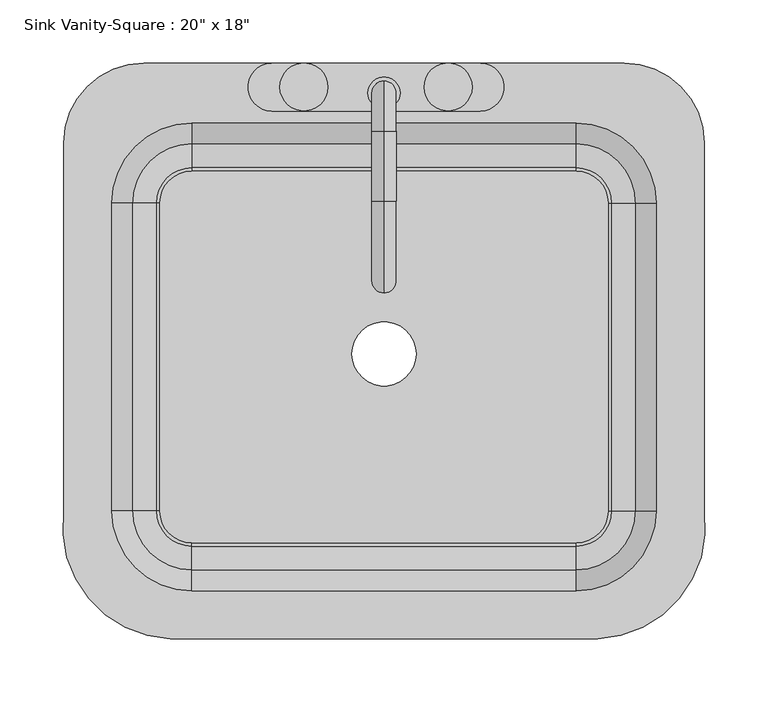
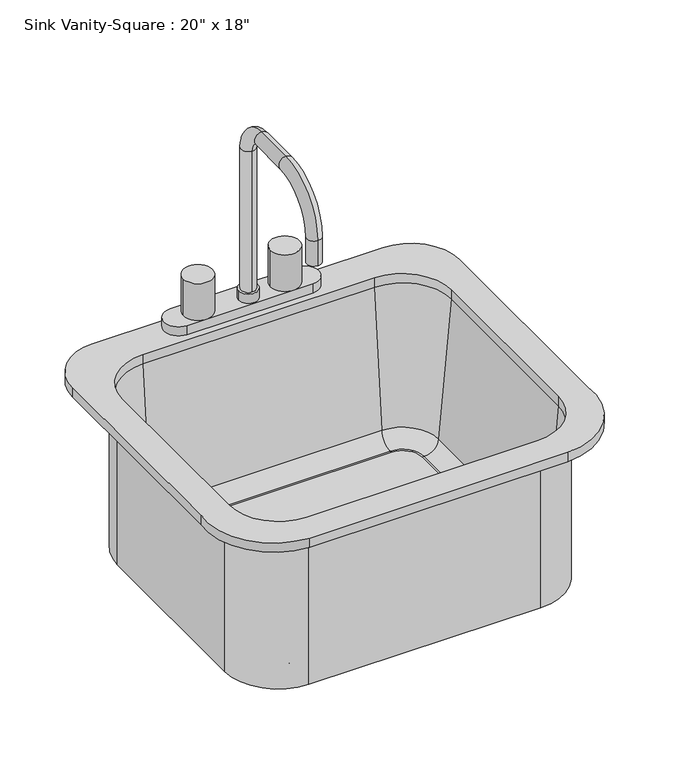
"""IFC4 building model written with IfcOpenShell, lengths in millimetres: flow terminal geometry."""

from ifc_helpers import new_model, si_unit, point, frame, frame_2d, origin, place, context, project, spatial, polyline, circle_curve, ellipse_curve, trimmed, segment, composite_curve, outline, extrude, source, transform, mapped, element, save
from ifc_brep_helpers import plane_surface, cylinder_surface, revolved_surface, advanced_brep


def flow_terminal_8d9ea526(model_context):
    return source(origin(), model_context, "Body", "SolidModel", [
        extrude(outline(composite_curve([segment(trimmed(circle_curve(frame_2d((168.0892406, 69.0204011)), 25.4), [point((168.0892406, 94.4204011))], [point((193.4892406, 69.0204011))], False, "CARTESIAN"), True, "CONTINUOUS"), segment(polyline([(193.4892406, 69.0204011), (193.4892406, -175.4545989)]), True, "CONTINUOUS"), segment(trimmed(circle_curve(frame_2d((168.0892406, -175.4545989)), 25.4), [point((193.4892406, -175.4545989))], [point((168.0892406, -200.8545989))], False, "CARTESIAN"), True, "CONTINUOUS"), segment(polyline([(168.0892406, -200.8545989), (-136.7107594, -200.8545989)]), True, "CONTINUOUS"), segment(trimmed(circle_curve(frame_2d((-136.7107594, -175.4545989)), 25.4), [point((-136.7107594, -200.8545989))], [point((-162.1107594, -175.4545989))], False, "CARTESIAN"), True, "CONTINUOUS"), segment(polyline([(-162.1107594, -175.4545989), (-162.1107594, 69.0204011)]), True, "CONTINUOUS"), segment(trimmed(circle_curve(frame_2d((-136.7107594, 69.0204011)), 25.4), [point((-162.1107594, 69.0204011))], [point((-136.7107594, 94.4204011))], False, "CARTESIAN"), True, "CONTINUOUS"), segment(polyline([(-136.7107594, 94.4204011), (168.0892406, 94.4204011)]), True, "CONTINUOUS")], self_intersect=False), holes=[composite_curve([segment(trimmed(circle_curve(frame_2d((15.6892406, -50.8)), 25.4), [point((-9.7107594, -50.8))], [point((41.0892406, -50.8))], True, "CARTESIAN"), True, "CONTINUOUS"), segment(trimmed(circle_curve(frame_2d((15.6892406, -50.8)), 25.4), [point((41.0892406, -50.8))], [point((-9.7107594, -50.8))], True, "CARTESIAN"), True, "CONTINUOUS")], self_intersect=False)]), frame((0.0, 0.0, 571.5), z_axis=(0.0, 0.0, 1.0), x_axis=(1.0, 0.0, 0.0)), (0.0, 0.0, 1.0), 9.525),
        extrude(outline(composite_curve([segment(trimmed(circle_curve(frame_2d((-47.8107594, 161.0954011)), 19.05), [point((-66.8607594, 161.0954011))], [point((-28.7607594, 161.0954011))], False, "CARTESIAN"), True, "CONTINUOUS"), segment(trimmed(circle_curve(frame_2d((-47.8107594, 161.0954011)), 19.05), [point((-28.7607594, 161.0954011))], [point((-66.8607594, 161.0954011))], False, "CARTESIAN"), True, "CONTINUOUS")], self_intersect=False)), frame((0.0, 0.0, 812.8), z_axis=(0.0, 0.0, 1.0), x_axis=(1.0, 0.0, 0.0)), (0.0, 0.0, 1.0), 50.8),
        extrude(outline(composite_curve([segment(trimmed(circle_curve(frame_2d((66.4892406, 161.0954011)), 19.05), [point((47.4392406, 161.0954011))], [point((85.5392406, 161.0954011))], False, "CARTESIAN"), True, "CONTINUOUS"), segment(trimmed(circle_curve(frame_2d((66.4892406, 161.0954011)), 19.05), [point((85.5392406, 161.0954011))], [point((47.4392406, 161.0954011))], False, "CARTESIAN"), True, "CONTINUOUS")], self_intersect=False)), frame((0.0, 0.0, 812.8), z_axis=(0.0, 0.0, 1.0), x_axis=(1.0, 0.0, 0.0)), (0.0, 0.0, 1.0), 50.8),
        advanced_brep(
        [(91.8892406, 180.1454011, 800.1), (91.8892406, 142.0454011, 800.1), (-73.2107594, 142.0454011, 800.1), (-73.2107594, 180.1454011, 800.1), (15.6892406, 165.8579011, 1020.7625), (15.6892406, 146.8079011, 1020.7625), (15.6892406, 146.8079011, 825.5), (15.6892406, 165.8579011, 825.5), (15.6892406, 126.1704011, 1060.45), (15.6892406, 126.1704011, 1041.4), (15.6892406, 70.6079011, 1060.45), (15.6892406, 70.6079011, 1041.4), (15.6892406, -2.4170989, 987.425), (15.6892406, 16.6329011, 987.425), (15.6892406, -2.4170989, 952.5), (15.6892406, 16.6329011, 952.5), (2.9892406, 156.3329011, 825.5), (28.3892406, 156.3329011, 825.5), (2.9892406, 156.3329011, 812.8), (28.3892406, 156.3329011, 812.8), (91.8892406, 180.1454011, 812.8), (-73.2107594, 180.1454011, 812.8), (-73.2107594, 142.0454011, 812.8), (91.8892406, 142.0454011, 812.8)],
        [
            (0, 1, circle_curve(frame((91.8892406, 161.0954011, 800.1), z_axis=(0.0, 0.0, -1.0), x_axis=(1.0, 0.0, 0.0)), 19.05)),
            (1, 2),
            (2, 3, circle_curve(frame((-73.2107594, 161.0954011, 800.1), z_axis=(0.0, 0.0, -1.0), x_axis=(1.0, 0.0, 0.0)), 19.05)),
            (3, 0),
            (4, 5, circle_curve(frame((15.6892406, 156.3329011, 1020.7625), z_axis=(0.0, 0.0, -1.0), x_axis=(0.0, -1.0, 0.0)), 9.525)),
            (5, 6),
            (6, 7, circle_curve(frame((15.6892406, 156.3329011, 825.5), z_axis=(0.0, 0.0, 1.0), x_axis=(0.0, -1.0, 0.0)), 9.525)),
            (7, 4),
            (5, 4, circle_curve(frame((15.6892406, 156.3329011, 1020.7625), z_axis=(0.0, 0.0, -1.0), x_axis=(0.0, -1.0, 0.0)), 9.525)),
            (7, 6, circle_curve(frame((15.6892406, 156.3329011, 825.5), z_axis=(0.0, 0.0, 1.0), x_axis=(0.0, -1.0, 0.0)), 9.525)),
            (4, 8, circle_curve(frame((15.6892406, 126.1704011, 1020.7625), z_axis=(1.0, 0.0, 0.0), x_axis=(0.0, 1.0, 0.0)), 39.6875)),
            (8, 9, circle_curve(frame((15.6892406, 126.1704011, 1050.925), z_axis=(0.0, 1.0, 0.0), x_axis=(0.0, 0.0, -1.0)), 9.525)),
            (9, 5, circle_curve(frame((15.6892406, 126.1704011, 1020.7625), z_axis=(-1.0, 0.0, 0.0), x_axis=(0.0, 1.0, 0.0)), 20.6375)),
            (9, 8, circle_curve(frame((15.6892406, 126.1704011, 1050.925), z_axis=(0.0, 1.0, 0.0), x_axis=(0.0, 0.0, -1.0)), 9.525)),
            (8, 10),
            (10, 11, circle_curve(frame((15.6892406, 70.6079011, 1050.925), z_axis=(0.0, 1.0, 0.0), x_axis=(0.0, 0.0, -1.0)), 9.525)),
            (11, 9),
            (11, 10, circle_curve(frame((15.6892406, 70.6079011, 1050.925), z_axis=(0.0, 1.0, 0.0), x_axis=(0.0, 0.0, -1.0)), 9.525)),
            (10, 12, circle_curve(frame((15.6892406, 70.6079011, 987.425), z_axis=(1.0, 0.0, 0.0), x_axis=(0.0, 0.0, 1.0)), 73.025)),
            (12, 13, circle_curve(frame((15.6892406, 7.1079011, 987.425), z_axis=(0.0, 0.0, 1.0), x_axis=(0.0, 1.0, 0.0)), 9.525)),
            (13, 11, circle_curve(frame((15.6892406, 70.6079011, 987.425), z_axis=(-1.0, 0.0, 0.0), x_axis=(0.0, 0.0, 1.0)), 53.975)),
            (13, 12, circle_curve(frame((15.6892406, 7.1079011, 987.425), z_axis=(0.0, 0.0, 1.0), x_axis=(0.0, 1.0, 0.0)), 9.525)),
            (14, 15, circle_curve(frame((15.6892406, 7.1079011, 952.5), z_axis=(0.0, 0.0, -1.0), x_axis=(0.0, 1.0, 0.0)), 9.525)),
            (15, 14, circle_curve(frame((15.6892406, 7.1079011, 952.5), z_axis=(0.0, 0.0, -1.0), x_axis=(0.0, 1.0, 0.0)), 9.525)),
            (12, 14),
            (15, 13),
            (16, 17, circle_curve(frame((15.6892406, 156.3329011, 825.5), z_axis=(0.0, 0.0, 1.0), x_axis=(1.0, 0.0, 0.0)), 12.7)),
            (17, 16, circle_curve(frame((15.6892406, 156.3329011, 825.5), z_axis=(0.0, 0.0, 1.0), x_axis=(1.0, 0.0, 0.0)), 12.7)),
            (16, 18),
            (18, 19, circle_curve(frame((15.6892406, 156.3329011, 812.8), z_axis=(0.0, 0.0, 1.0), x_axis=(1.0, 0.0, 0.0)), 12.7)),
            (19, 17),
            (19, 18, circle_curve(frame((15.6892406, 156.3329011, 812.8), z_axis=(0.0, 0.0, 1.0), x_axis=(1.0, 0.0, 0.0)), 12.7)),
            (20, 21),
            (21, 22, circle_curve(frame((-73.2107594, 161.0954011, 812.8), z_axis=(0.0, 0.0, 1.0), x_axis=(1.0, 0.0, 0.0)), 19.05)),
            (22, 23),
            (23, 20, circle_curve(frame((91.8892406, 161.0954011, 812.8), z_axis=(0.0, 0.0, 1.0), x_axis=(1.0, 0.0, 0.0)), 19.05)),
            (20, 0),
            (3, 21),
            (2, 22),
            (1, 23),
        ],
        [
            plane_surface(frame((15.6892406, 146.8079011, 800.1), z_axis=(0.0, 0.0, -1.0), x_axis=(1.0, 0.0, 0.0))),
            cylinder_surface(frame((15.6892406, 156.3329011, 800.1), z_axis=(0.0, 0.0, -1.0), x_axis=(0.0, -1.0, 0.0)), 9.525),
            revolved_surface(trimmed(ellipse_curve(frame((15.6892406, 156.3329011, 1020.7625), z_axis=(0.0, 0.0, -1.0), x_axis=(0.0, -1.0, 0.0)), 9.525, 9.525), [point((15.6892406, 165.8579011, 1020.7625))], [point((15.6892406, 146.8079011, 1020.7625))], True, "CARTESIAN"), (15.6892406, 126.1704011, 1020.7625), (1.0, 0.0, 0.0)),
            revolved_surface(trimmed(ellipse_curve(frame((15.6892406, 156.3329011, 1020.7625), z_axis=(0.0, 0.0, -1.0), x_axis=(0.0, -1.0, 0.0)), 9.525, 9.525), [point((15.6892406, 146.8079011, 1020.7625))], [point((15.6892406, 165.8579011, 1020.7625))], True, "CARTESIAN"), (15.6892406, 126.1704011, 1020.7625), (1.0, 0.0, 0.0)),
            cylinder_surface(frame((15.6892406, 126.1704011, 1050.925), z_axis=(0.0, 1.0, 0.0), x_axis=(0.0, 0.0, -1.0)), 9.525),
            revolved_surface(trimmed(ellipse_curve(frame((15.6892406, 70.6079011, 1050.925), z_axis=(0.0, 1.0, 0.0), x_axis=(0.0, 0.0, -1.0)), 9.525, 9.525), [point((15.6892406, 70.6079011, 1060.45))], [point((15.6892406, 70.6079011, 1041.4))], True, "CARTESIAN"), (15.6892406, 70.6079011, 987.425), (1.0, 0.0, 0.0)),
            revolved_surface(trimmed(ellipse_curve(frame((15.6892406, 70.6079011, 1050.925), z_axis=(0.0, 1.0, 0.0), x_axis=(0.0, 0.0, -1.0)), 9.525, 9.525), [point((15.6892406, 70.6079011, 1041.4))], [point((15.6892406, 70.6079011, 1060.45))], True, "CARTESIAN"), (15.6892406, 70.6079011, 987.425), (1.0, 0.0, 0.0)),
            plane_surface(frame((15.6892406, -2.4170989, 952.5), z_axis=(0.0, 0.0, -1.0), x_axis=(-1.0, 0.0, 0.0))),
            cylinder_surface(frame((15.6892406, 7.1079011, 987.425), z_axis=(0.0, 0.0, 1.0), x_axis=(0.0, 1.0, 0.0)), 9.525),
            plane_surface(frame((28.3892406, 156.3329011, 825.5), z_axis=(0.0, 0.0, 1.0), x_axis=(0.0, 1.0, 0.0))),
            cylinder_surface(frame((15.6892406, 156.3329011, 812.8), z_axis=(0.0, 0.0, 1.0), x_axis=(1.0, 0.0, 0.0)), 12.7),
            plane_surface(frame((-73.2107594, 180.1454011, 812.8), z_axis=(0.0, 0.0, 1.0), x_axis=(-1.0, 0.0, 0.0))),
            plane_surface(frame((91.8892406, 180.1454011, 812.8), z_axis=(0.0, 1.0, 0.0), x_axis=(0.0, 0.0, -1.0))),
            cylinder_surface(frame((-73.2107594, 161.0954011, 800.1), z_axis=(0.0, 0.0, 1.0), x_axis=(1.0, 0.0, 0.0)), 19.05),
            plane_surface(frame((-73.2107594, 142.0454011, 812.8), z_axis=(0.0, -1.0, 0.0), x_axis=(0.0, 0.0, -1.0))),
            cylinder_surface(frame((91.8892406, 161.0954011, 800.1), z_axis=(0.0, 0.0, 1.0), x_axis=(1.0, 0.0, 0.0)), 19.05),
        ],
        [
            (0, [[1, 2, 3, 4]]),
            (1, [[5, 6, 7, 8]]),
            (1, [[9, -8, 10, -6]]),
            (2, [[-5, 11, 12, 13]]),
            (3, [[-9, -13, 14, -11]]),
            (4, [[-12, 15, 16, 17]]),
            (4, [[-14, -17, 18, -15]]),
            (5, [[-16, 19, 20, 21]]),
            (6, [[-18, -21, 22, -19]]),
            (7, [[23, 24]]),
            (8, [[-20, 25, -24, 26]]),
            (8, [[-22, -26, -23, -25]]),
            (9, [[27, 28], [-7, -10]]),
            (10, [[-27, 29, 30, 31]]),
            (10, [[-28, -31, 32, -29]]),
            (11, [[33, 34, 35, 36], [-30, -32]]),
            (12, [[-33, 37, -4, 38]]),
            (13, [[-34, -38, -3, 39]]),
            (14, [[-35, -39, -2, 40]]),
            (15, [[-36, -40, -1, -37]]),
        ],
    ),
        advanced_brep(
        [(-153.9606923, -277.0545989, 800.1), (185.3391735, -277.0545989, 800.1), (269.6892406, -175.4545989, 800.1), (269.6892406, 116.6454011, 800.1), (206.1892406, 180.1454011, 800.1), (-174.8107593, 180.1454011, 800.1), (-238.3107593, 116.6454011, 800.1), (-238.3107593, -175.4545982, 800.1), (168.0892406, 132.5204011, 800.1), (231.5892406, 69.0204011, 800.1), (231.5892406, -175.4545989, 800.1), (168.0892406, -238.9545989, 800.1), (-136.7107594, -238.9545989, 800.1), (-200.2107594, -175.4545989, 800.1), (-200.2107594, 69.0204011, 800.1), (-136.7107594, 132.5204011, 800.1), (-153.9606923, -277.0545989, 787.4), (-238.3107593, -175.4545982, 787.4), (-238.3107593, 116.6454011, 787.4), (-174.8107593, 180.1454011, 787.4), (206.1892406, 180.1454011, 787.4), (269.6892406, 116.6454011, 787.4), (269.6892406, -175.4545989, 787.4), (185.3391735, -277.0545989, 787.4), (237.9392406, 69.0204011, 787.4), (168.0892406, 138.8704011, 787.4), (-136.7107594, 138.8704011, 787.4), (-206.5607594, 69.0204011, 787.4), (-206.5607594, -175.4545989, 787.4), (-136.7107594, -245.3045989, 787.4), (168.0892406, -245.3045989, 787.4), (237.9392406, -175.4545989, 787.4), (168.0892406, 132.5204011, 787.4), (231.5892406, 69.0204011, 787.4), (231.5892406, -175.4545989, 787.4), (168.0892406, -238.9545989, 787.4), (-136.7107594, -238.9545989, 787.4), (-200.2107594, -175.4545989, 787.4), (-200.2107594, 69.0204011, 787.4), (-136.7107594, 132.5204011, 787.4), (237.9392406, 69.0204011, 571.5), (168.0892406, 138.8704011, 571.5), (193.4892406, 69.0204011, 571.5), (168.0892406, 94.4204011, 571.5), (193.4892406, 69.0204011, 581.025), (168.0892406, 94.4204011, 581.025), (196.0776588, 69.0204011, 581.025), (168.0892406, 97.0088193, 581.025), (215.0551678, 69.0204011, 598.4146831), (168.0892406, 115.9863283, 598.4146831), (237.9392406, -175.4545989, 571.5), (193.4892406, -175.4545989, 571.5), (193.4892406, -175.4545989, 581.025), (196.0776588, -175.4545989, 581.025), (215.0551678, -175.4545989, 598.4146831), (168.0892406, -245.3045989, 571.5), (168.0892406, -200.8545989, 571.5), (168.0892406, -200.8545989, 581.025), (168.0892406, -203.4430171, 581.025), (168.0892406, -222.4205261, 598.4146831), (-136.7107594, -245.3045989, 571.5), (-136.7107594, -200.8545989, 571.5), (-136.7107594, -200.8545989, 581.025), (-136.7107594, -203.4430171, 581.025), (-136.7107594, -222.4205261, 598.4146831), (-206.5607594, -175.4545989, 571.5), (-162.1107594, -175.4545989, 571.5), (-162.1107594, -175.4545989, 581.025), (-164.6991776, -175.4545989, 581.025), (-183.6766866, -175.4545989, 598.4146831), (-206.5607594, 69.0204011, 571.5), (-162.1107594, 69.0204011, 571.5), (-162.1107594, 69.0204011, 581.025), (-164.6991776, 69.0204011, 581.025), (-183.6766866, 69.0204011, 598.4146831), (-136.7107594, 138.8704011, 571.5), (-136.7107594, 94.4204011, 571.5), (-136.7107594, 94.4204011, 581.025), (-136.7107594, 97.0088193, 581.025), (-136.7107594, 115.9863283, 598.4146831)],
        [
            (0, 1),
            (1, 2, circle_curve(frame((181.5319557, -188.0793432, 800.1), z_axis=(0.0, 0.0, 1.0), x_axis=(1.0, 0.0, 0.0)), 89.0566732)),
            (2, 3),
            (3, 4, circle_curve(frame((206.1892406, 116.6454011, 800.1), z_axis=(0.0, 0.0, 1.0), x_axis=(1.0, 0.0, 0.0)), 63.5)),
            (4, 5),
            (5, 6, circle_curve(frame((-174.8107593, 116.6454011, 800.1), z_axis=(0.0, 0.0, 1.0), x_axis=(1.0, 0.0, 0.0)), 63.5)),
            (6, 7),
            (7, 0, circle_curve(frame((-150.1534746, -188.0793432, 800.1), z_axis=(0.0, 0.0, 1.0), x_axis=(1.0, 0.0, 0.0)), 89.0566732)),
            (8, 9, circle_curve(frame((168.0892406, 69.0204011, 800.1), z_axis=(0.0, 0.0, -1.0), x_axis=(1.0, 0.0, 0.0)), 63.5)),
            (9, 10),
            (10, 11, circle_curve(frame((168.0892406, -175.4545989, 800.1), z_axis=(0.0, 0.0, -1.0), x_axis=(1.0, 0.0, 0.0)), 63.5)),
            (11, 12),
            (12, 13, circle_curve(frame((-136.7107594, -175.4545989, 800.1), z_axis=(0.0, 0.0, -1.0), x_axis=(1.0, 0.0, 0.0)), 63.5)),
            (13, 14),
            (14, 15, circle_curve(frame((-136.7107594, 69.0204011, 800.1), z_axis=(0.0, 0.0, -1.0), x_axis=(1.0, 0.0, 0.0)), 63.5)),
            (15, 8),
            (16, 17, circle_curve(frame((-150.1534746, -188.0793432, 787.4), z_axis=(0.0, 0.0, -1.0), x_axis=(1.0, 0.0, 0.0)), 89.0566732)),
            (17, 18),
            (18, 19, circle_curve(frame((-174.8107593, 116.6454011, 787.4), z_axis=(0.0, 0.0, -1.0), x_axis=(1.0, 0.0, 0.0)), 63.5)),
            (19, 20),
            (20, 21, circle_curve(frame((206.1892406, 116.6454011, 787.4), z_axis=(0.0, 0.0, -1.0), x_axis=(1.0, 0.0, 0.0)), 63.5)),
            (21, 22),
            (22, 23, circle_curve(frame((181.5319557, -188.0793432, 787.4), z_axis=(0.0, 0.0, -1.0), x_axis=(1.0, 0.0, 0.0)), 89.0566732)),
            (23, 16),
            (24, 25, circle_curve(frame((168.0892406, 69.0204011, 787.4), z_axis=(0.0, 0.0, 1.0), x_axis=(0.0, 1.0, 0.0)), 69.85)),
            (25, 26),
            (26, 27, circle_curve(frame((-136.7107594, 69.0204011, 787.4), z_axis=(0.0, 0.0, 1.0), x_axis=(-1.0, 0.0, 0.0)), 69.85)),
            (27, 28),
            (28, 29, circle_curve(frame((-136.7107594, -175.4545989, 787.4), z_axis=(0.0, 0.0, 1.0), x_axis=(0.0, -1.0, 0.0)), 69.85)),
            (29, 30),
            (30, 31, circle_curve(frame((168.0892406, -175.4545989, 787.4), z_axis=(0.0, 0.0, 1.0), x_axis=(1.0, 0.0, 0.0)), 69.85)),
            (31, 24),
            (0, 16),
            (23, 1),
            (22, 2),
            (21, 3),
            (20, 4),
            (19, 5),
            (18, 6),
            (17, 7),
            (8, 32),
            (32, 33, circle_curve(frame((168.0892406, 69.0204011, 787.4), z_axis=(0.0, 0.0, -1.0), x_axis=(1.0, 0.0, 0.0)), 63.5)),
            (33, 9),
            (33, 34),
            (34, 10),
            (34, 35, circle_curve(frame((168.0892406, -175.4545989, 787.4), z_axis=(0.0, 0.0, -1.0), x_axis=(1.0, 0.0, 0.0)), 63.5)),
            (35, 11),
            (35, 36),
            (36, 12),
            (36, 37, circle_curve(frame((-136.7107594, -175.4545989, 787.4), z_axis=(0.0, 0.0, -1.0), x_axis=(1.0, 0.0, 0.0)), 63.5)),
            (37, 13),
            (37, 38),
            (38, 14),
            (38, 39, circle_curve(frame((-136.7107594, 69.0204011, 787.4), z_axis=(0.0, 0.0, -1.0), x_axis=(1.0, 0.0, 0.0)), 63.5)),
            (39, 15),
            (39, 32),
            (40, 41, circle_curve(frame((168.0892406, 69.0204011, 571.5), z_axis=(0.0, 0.0, 1.0), x_axis=(0.0, 1.0, 0.0)), 69.85)),
            (41, 25),
            (24, 40),
            (40, 42),
            (42, 43, circle_curve(frame((168.0892406, 69.0204011, 571.5), z_axis=(0.0, 0.0, 1.0), x_axis=(0.0, 1.0, 0.0)), 25.4)),
            (43, 41),
            (42, 44),
            (44, 45, circle_curve(frame((168.0892406, 69.0204011, 581.025), z_axis=(0.0, 0.0, 1.0), x_axis=(0.0, 1.0, 0.0)), 25.4)),
            (45, 43),
            (44, 46),
            (46, 47, circle_curve(frame((168.0892406, 69.0204011, 581.025), z_axis=(0.0, 0.0, 1.0), x_axis=(0.0, 1.0, 0.0)), 27.9884182)),
            (47, 45),
            (46, 48, circle_curve(frame((196.0776588, 69.0204011, 600.075), z_axis=(0.0, -1.0, 0.0), x_axis=(1.0, 0.0, 0.0)), 19.05)),
            (48, 49, circle_curve(frame((168.0892406, 69.0204011, 598.4146831), z_axis=(0.0, 0.0, 1.0), x_axis=(0.0, 1.0, 0.0)), 46.9659272)),
            (49, 47, circle_curve(frame((168.0892406, 97.0088193, 600.075), z_axis=(-1.0, 0.0, 0.0), x_axis=(0.0, 1.0, 0.0)), 19.05)),
            (48, 33),
            (32, 49),
            (31, 50),
            (50, 40),
            (50, 51),
            (51, 42),
            (51, 52),
            (52, 44),
            (52, 53),
            (53, 46),
            (53, 54, circle_curve(frame((196.0776588, -175.4545989, 600.075), z_axis=(0.0, -1.0, 0.0), x_axis=(1.0, 0.0, 0.0)), 19.05)),
            (54, 48),
            (54, 34),
            (30, 55),
            (55, 50, circle_curve(frame((168.0892406, -175.4545989, 571.5), z_axis=(0.0, 0.0, 1.0), x_axis=(1.0, 0.0, 0.0)), 69.85)),
            (55, 56),
            (56, 51, circle_curve(frame((168.0892406, -175.4545989, 571.5), z_axis=(0.0, 0.0, 1.0), x_axis=(1.0, 0.0, 0.0)), 25.4)),
            (56, 57),
            (57, 52, circle_curve(frame((168.0892406, -175.4545989, 581.025), z_axis=(0.0, 0.0, 1.0), x_axis=(1.0, 0.0, 0.0)), 25.4)),
            (57, 58),
            (58, 53, circle_curve(frame((168.0892406, -175.4545989, 581.025), z_axis=(0.0, 0.0, 1.0), x_axis=(1.0, 0.0, 0.0)), 27.9884182)),
            (58, 59, circle_curve(frame((168.0892406, -203.4430171, 600.075), z_axis=(-1.0, 0.0, 0.0), x_axis=(0.0, -1.0, 0.0)), 19.05)),
            (59, 54, circle_curve(frame((168.0892406, -175.4545989, 598.4146831), z_axis=(0.0, 0.0, 1.0), x_axis=(1.0, 0.0, 0.0)), 46.9659272)),
            (59, 35),
            (29, 60),
            (60, 55),
            (60, 61),
            (61, 56),
            (61, 62),
            (62, 57),
            (62, 63),
            (63, 58),
            (63, 64, circle_curve(frame((-136.7107594, -203.4430171, 600.075), z_axis=(-1.0, 0.0, 0.0), x_axis=(0.0, -1.0, 0.0)), 19.05)),
            (64, 59),
            (64, 36),
            (28, 65),
            (65, 60, circle_curve(frame((-136.7107594, -175.4545989, 571.5), z_axis=(0.0, 0.0, 1.0), x_axis=(0.0, -1.0, 0.0)), 69.85)),
            (65, 66),
            (66, 61, circle_curve(frame((-136.7107594, -175.4545989, 571.5), z_axis=(0.0, 0.0, 1.0), x_axis=(0.0, -1.0, 0.0)), 25.4)),
            (66, 67),
            (67, 62, circle_curve(frame((-136.7107594, -175.4545989, 581.025), z_axis=(0.0, 0.0, 1.0), x_axis=(0.0, -1.0, 0.0)), 25.4)),
            (67, 68),
            (68, 63, circle_curve(frame((-136.7107594, -175.4545989, 581.025), z_axis=(0.0, 0.0, 1.0), x_axis=(0.0, -1.0, 0.0)), 27.9884182)),
            (68, 69, circle_curve(frame((-164.6991776, -175.4545989, 600.075), z_axis=(0.0, 1.0, 0.0), x_axis=(-1.0, 0.0, 0.0)), 19.05)),
            (69, 64, circle_curve(frame((-136.7107594, -175.4545989, 598.4146831), z_axis=(0.0, 0.0, 1.0), x_axis=(0.0, -1.0, 0.0)), 46.9659272)),
            (69, 37),
            (27, 70),
            (70, 65),
            (70, 71),
            (71, 66),
            (71, 72),
            (72, 67),
            (72, 73),
            (73, 68),
            (73, 74, circle_curve(frame((-164.6991776, 69.0204011, 600.075), z_axis=(0.0, 1.0, 0.0), x_axis=(-1.0, 0.0, 0.0)), 19.05)),
            (74, 69),
            (74, 38),
            (26, 75),
            (75, 70, circle_curve(frame((-136.7107594, 69.0204011, 571.5), z_axis=(0.0, 0.0, 1.0), x_axis=(-1.0, 0.0, 0.0)), 69.85)),
            (75, 76),
            (76, 71, circle_curve(frame((-136.7107594, 69.0204011, 571.5), z_axis=(0.0, 0.0, 1.0), x_axis=(-1.0, 0.0, 0.0)), 25.4)),
            (76, 77),
            (77, 72, circle_curve(frame((-136.7107594, 69.0204011, 581.025), z_axis=(0.0, 0.0, 1.0), x_axis=(-1.0, 0.0, 0.0)), 25.4)),
            (77, 78),
            (78, 73, circle_curve(frame((-136.7107594, 69.0204011, 581.025), z_axis=(0.0, 0.0, 1.0), x_axis=(-1.0, 0.0, 0.0)), 27.9884182)),
            (78, 79, circle_curve(frame((-136.7107594, 97.0088193, 600.075), z_axis=(1.0, 0.0, 0.0), x_axis=(0.0, 1.0, 0.0)), 19.05)),
            (79, 74, circle_curve(frame((-136.7107594, 69.0204011, 598.4146831), z_axis=(0.0, 0.0, 1.0), x_axis=(-1.0, 0.0, 0.0)), 46.9659272)),
            (79, 39),
            (41, 75),
            (43, 76),
            (45, 77),
            (47, 78),
            (49, 79),
        ],
        [
            plane_surface(frame((185.3391735, -277.0545989, 800.1), z_axis=(0.0, 0.0, 1.0), x_axis=(1.0, 0.0, 0.0))),
            plane_surface(frame((185.3391735, -277.0545989, 787.4), z_axis=(0.0, 0.0, -1.0), x_axis=(-1.0, 0.0, 0.0))),
            plane_surface(frame((-153.9606923, -277.0545989, 800.1), z_axis=(0.0, -1.0, 0.0), x_axis=(0.0, 0.0, -1.0))),
            cylinder_surface(frame((181.5319557, -188.0793432, 787.4), z_axis=(0.0, 0.0, 1.0), x_axis=(1.0, 0.0, 0.0)), 89.0566732),
            plane_surface(frame((269.6892406, -175.4545989, 800.1), z_axis=(1.0, 0.0, 0.0), x_axis=(0.0, 0.0, -1.0))),
            cylinder_surface(frame((206.1892406, 116.6454011, 787.4), z_axis=(0.0, 0.0, 1.0), x_axis=(1.0, 0.0, 0.0)), 63.5),
            plane_surface(frame((206.1892406, 180.1454011, 800.1), z_axis=(0.0, 1.0, 0.0), x_axis=(0.0, 0.0, -1.0))),
            cylinder_surface(frame((-174.8107593, 116.6454011, 787.4), z_axis=(0.0, 0.0, 1.0), x_axis=(1.0, 0.0, 0.0)), 63.5),
            plane_surface(frame((-238.3107593, 116.6454011, 800.1), z_axis=(-1.0, 0.0, 0.0), x_axis=(0.0, 0.0, -1.0))),
            cylinder_surface(frame((-150.1534746, -188.0793432, 787.4), z_axis=(0.0, 0.0, 1.0), x_axis=(1.0, 0.0, 0.0)), 89.0566732),
            revolved_surface(polyline([(231.5892406, 69.0204011, 787.4), (231.5892406, 69.0204011, 800.1)]), (168.0892406, 69.0204011, 0.0), (0.0, 0.0, -1.0)),
            plane_surface(frame((231.5892406, 69.0204011, 800.1), z_axis=(-1.0, 0.0, 0.0), x_axis=(0.0, 0.0, -1.0))),
            revolved_surface(polyline([(231.5892406, -175.4545989, 787.4), (231.5892406, -175.4545989, 800.1)]), (168.0892406, -175.4545989, 0.0), (0.0, 0.0, -1.0)),
            plane_surface(frame((168.0892406, -238.9545989, 800.1), z_axis=(0.0, 1.0, 0.0), x_axis=(0.0, 0.0, -1.0))),
            revolved_surface(polyline([(-73.2107594, -175.4545989, 787.4), (-73.2107594, -175.4545989, 800.1)]), (-136.7107594, -175.4545989, 0.0), (0.0, 0.0, -1.0)),
            plane_surface(frame((-200.2107594, -175.4545989, 800.1), z_axis=(1.0, 0.0, 0.0), x_axis=(0.0, 0.0, -1.0))),
            revolved_surface(polyline([(-73.2107594, 69.0204011, 787.4), (-73.2107594, 69.0204011, 800.1)]), (-136.7107594, 69.0204011, 0.0), (0.0, 0.0, -1.0)),
            plane_surface(frame((-136.7107594, 132.5204011, 800.1), z_axis=(0.0, -1.0, 0.0), x_axis=(0.0, 0.0, -1.0))),
            cylinder_surface(frame((168.0892406, 69.0204011, 0.0), z_axis=(0.0, 0.0, -1.0), x_axis=(0.0, 1.0, 0.0)), 69.85),
            plane_surface(frame((168.0892406, 69.0204011, 571.5), z_axis=(0.0, 0.0, -1.0), x_axis=(0.0, 1.0, 0.0))),
            revolved_surface(polyline([(168.0892406, 94.42040109999999, 571.5), (168.0892406, 94.42040109999999, 581.025)]), (168.0892406, 69.0204011, 0.0), (0.0, 0.0, -1.0)),
            plane_surface(frame((168.0892406, 69.0204011, 581.025), z_axis=(0.0, 0.0, 1.0), x_axis=(0.0, 1.0, 0.0))),
            revolved_surface(trimmed(ellipse_curve(frame((168.0892406, 97.0088193, 600.075), z_axis=(1.0, 0.0, 0.0), x_axis=(0.0, 1.0, 0.0)), 19.05, 19.05), [point((168.0892406, 97.0088193, 581.025))], [point((168.0892406, 115.9863283, 598.4146831))], True, "CARTESIAN"), (168.0892406, 69.0204011, 0.0), (0.0, 0.0, -1.0)),
            revolved_surface(polyline([(168.0892406, 115.9863283, 598.4146831), (168.0892406, 132.5204011, 787.4)]), (168.0892406, 69.0204011, 0.0), (0.0, 0.0, -1.0)),
            plane_surface(frame((237.9392406, 69.0204011, 787.4), z_axis=(1.0, 0.0, 0.0), x_axis=(0.0, -1.0, 0.0))),
            plane_surface(frame((237.9392406, 69.0204011, 571.5), z_axis=(0.0, 0.0, -1.0), x_axis=(0.0, -1.0, 0.0))),
            plane_surface(frame((193.4892406, 69.0204011, 571.5), z_axis=(-1.0, 0.0, 0.0), x_axis=(0.0, -1.0, 0.0))),
            plane_surface(frame((193.4892406, 69.0204011, 581.025), z_axis=(0.0, 0.0, 1.0), x_axis=(0.0, -1.0, 0.0))),
            revolved_surface(polyline([(215.1276588, -175.4545989, 600.075), (215.1276588, 69.0204011, 600.075)]), (196.0776588, 69.0204011, 600.075), (0.0, -1.0, 0.0)),
            plane_surface(frame((215.0551678, 69.0204011, 598.4146831), z_axis=(-0.9961946980917442, 0.0, 0.08715574274767397), x_axis=(0.0, -1.0, 0.0))),
            cylinder_surface(frame((168.0892406, -175.4545989, 0.0), z_axis=(0.0, 0.0, -1.0), x_axis=(1.0, 0.0, 0.0)), 69.85),
            plane_surface(frame((168.0892406, -175.4545989, 571.5), z_axis=(0.0, 0.0, -1.0), x_axis=(1.0, 0.0, 0.0))),
            revolved_surface(polyline([(193.48924060000002, -175.4545989, 571.5), (193.48924060000002, -175.4545989, 581.025)]), (168.0892406, -175.4545989, 0.0), (0.0, 0.0, -1.0)),
            plane_surface(frame((168.0892406, -175.4545989, 581.025), z_axis=(0.0, 0.0, 1.0), x_axis=(1.0, 0.0, 0.0))),
            revolved_surface(trimmed(ellipse_curve(frame((196.0776588, -175.4545989, 600.075), z_axis=(0.0, -1.0, 0.0), x_axis=(1.0, 0.0, 0.0)), 19.05, 19.05), [point((196.0776588, -175.4545989, 581.025))], [point((215.0551678, -175.4545989, 598.4146831))], True, "CARTESIAN"), (168.0892406, -175.4545989, 0.0), (0.0, 0.0, -1.0)),
            revolved_surface(polyline([(215.0551678, -175.4545989, 598.4146831), (231.5892406, -175.4545989, 787.4)]), (168.0892406, -175.4545989, 0.0), (0.0, 0.0, -1.0)),
            plane_surface(frame((168.0892406, -245.3045989, 787.4), z_axis=(0.0, -1.0, 0.0), x_axis=(-1.0, 0.0, 0.0))),
            plane_surface(frame((168.0892406, -245.3045989, 571.5), z_axis=(0.0, 0.0, -1.0), x_axis=(-1.0, 0.0, 0.0))),
            plane_surface(frame((168.0892406, -200.8545989, 571.5), z_axis=(0.0, 1.0, 0.0), x_axis=(-1.0, 0.0, 0.0))),
            plane_surface(frame((168.0892406, -200.8545989, 581.025), z_axis=(0.0, 0.0, 1.0), x_axis=(-1.0, 0.0, 0.0))),
            revolved_surface(polyline([(-136.7107594, -222.4930171, 600.075), (168.0892406, -222.4930171, 600.075)]), (168.0892406, -203.4430171, 600.075), (-1.0, 0.0, 0.0)),
            plane_surface(frame((168.0892406, -222.4205261, 598.4146831), z_axis=(0.0, 0.9961946980917442, 0.08715574274767397), x_axis=(-1.0, 0.0, 0.0))),
            cylinder_surface(frame((-136.7107594, -175.4545989, 0.0), z_axis=(0.0, 0.0, -1.0), x_axis=(0.0, -1.0, 0.0)), 69.85),
            plane_surface(frame((-136.7107594, -175.4545989, 571.5), z_axis=(0.0, 0.0, -1.0), x_axis=(0.0, -1.0, 0.0))),
            revolved_surface(polyline([(-136.7107594, -200.8545989, 571.5), (-136.7107594, -200.8545989, 581.025)]), (-136.7107594, -175.4545989, 0.0), (0.0, 0.0, -1.0)),
            plane_surface(frame((-136.7107594, -175.4545989, 581.025), z_axis=(0.0, 0.0, 1.0), x_axis=(0.0, -1.0, 0.0))),
            revolved_surface(trimmed(ellipse_curve(frame((-136.7107594, -203.4430171, 600.075), z_axis=(-1.0, 0.0, 0.0), x_axis=(0.0, -1.0, 0.0)), 19.05, 19.05), [point((-136.7107594, -203.4430171, 581.025))], [point((-136.7107594, -222.4205261, 598.4146831))], True, "CARTESIAN"), (-136.7107594, -175.4545989, 0.0), (0.0, 0.0, -1.0)),
            revolved_surface(polyline([(-136.7107594, -222.4205261, 598.4146831), (-136.7107594, -238.9545989, 787.4)]), (-136.7107594, -175.4545989, 0.0), (0.0, 0.0, -1.0)),
            plane_surface(frame((-206.5607594, -175.4545989, 787.4), z_axis=(-1.0, 0.0, 0.0), x_axis=(0.0, 1.0, 0.0))),
            plane_surface(frame((-206.5607594, -175.4545989, 571.5), z_axis=(0.0, 0.0, -1.0), x_axis=(0.0, 1.0, 0.0))),
            plane_surface(frame((-162.1107594, -175.4545989, 571.5), z_axis=(1.0, 0.0, 0.0), x_axis=(0.0, 1.0, 0.0))),
            plane_surface(frame((-162.1107594, -175.4545989, 581.025), z_axis=(0.0, 0.0, 1.0), x_axis=(0.0, 1.0, 0.0))),
            revolved_surface(polyline([(-183.74917760000002, 69.02040110000002, 600.075), (-183.74917760000002, -175.4545989, 600.075)]), (-164.6991776, -175.4545989, 600.075), (0.0, 1.0, 0.0)),
            plane_surface(frame((-183.6766866, -175.4545989, 598.4146831), z_axis=(0.9961946980917442, 0.0, 0.08715574274767397), x_axis=(0.0, 1.0, 0.0))),
            cylinder_surface(frame((-136.7107594, 69.0204011, 0.0), z_axis=(0.0, 0.0, -1.0), x_axis=(-1.0, 0.0, 0.0)), 69.85),
            plane_surface(frame((-136.7107594, 69.0204011, 571.5), z_axis=(0.0, 0.0, -1.0), x_axis=(-1.0, 0.0, 0.0))),
            revolved_surface(polyline([(-162.1107594, 69.0204011, 571.5), (-162.1107594, 69.0204011, 581.025)]), (-136.7107594, 69.0204011, 0.0), (0.0, 0.0, -1.0)),
            plane_surface(frame((-136.7107594, 69.0204011, 581.025), z_axis=(0.0, 0.0, 1.0), x_axis=(-1.0, 0.0, 0.0))),
            revolved_surface(trimmed(ellipse_curve(frame((-164.6991776, 69.0204011, 600.075), z_axis=(0.0, 1.0, 0.0), x_axis=(-1.0, 0.0, 0.0)), 19.05, 19.05), [point((-164.6991776, 69.0204011, 581.025))], [point((-183.6766866, 69.0204011, 598.4146831))], True, "CARTESIAN"), (-136.7107594, 69.0204011, 0.0), (0.0, 0.0, -1.0)),
            revolved_surface(polyline([(-183.6766866, 69.0204011, 598.4146831), (-200.2107594, 69.0204011, 787.4)]), (-136.7107594, 69.0204011, 0.0), (0.0, 0.0, -1.0)),
            plane_surface(frame((-136.7107594, 138.8704011, 787.4), z_axis=(0.0, 1.0, 0.0), x_axis=(1.0, 0.0, 0.0))),
            plane_surface(frame((-136.7107594, 138.8704011, 571.5), z_axis=(0.0, 0.0, -1.0), x_axis=(1.0, 0.0, 0.0))),
            plane_surface(frame((-136.7107594, 94.4204011, 571.5), z_axis=(0.0, -1.0, 0.0), x_axis=(1.0, 0.0, 0.0))),
            plane_surface(frame((-136.7107594, 94.4204011, 581.025), z_axis=(0.0, 0.0, 1.0), x_axis=(1.0, 0.0, 0.0))),
            revolved_surface(polyline([(168.0892406, 116.0588193, 600.075), (-136.7107594, 116.0588193, 600.075)]), (-136.7107594, 97.0088193, 600.075), (1.0, 0.0, 0.0)),
            plane_surface(frame((-136.7107594, 115.9863283, 598.4146831), z_axis=(0.0, -0.9961946980917442, 0.08715574274767397), x_axis=(1.0, 0.0, 0.0))),
        ],
        [
            (0, [[1, 2, 3, 4, 5, 6, 7, 8], [9, 10, 11, 12, 13, 14, 15, 16]]),
            (1, [[17, 18, 19, 20, 21, 22, 23, 24], [25, 26, 27, 28, 29, 30, 31, 32]]),
            (2, [[-1, 33, -24, 34]]),
            (3, [[-2, -34, -23, 35]]),
            (4, [[-3, -35, -22, 36]]),
            (5, [[-4, -36, -21, 37]]),
            (6, [[-5, -37, -20, 38]]),
            (7, [[-6, -38, -19, 39]]),
            (8, [[-7, -39, -18, 40]]),
            (9, [[-8, -40, -17, -33]]),
            (10, [[-9, 41, 42, 43]]),
            (11, [[-10, -43, 44, 45]]),
            (12, [[-11, -45, 46, 47]]),
            (13, [[-12, -47, 48, 49]]),
            (14, [[-13, -49, 50, 51]]),
            (15, [[-14, -51, 52, 53]]),
            (16, [[-15, -53, 54, 55]]),
            (17, [[-16, -55, 56, -41]]),
            (18, [[57, 58, -25, 59]]),
            (19, [[-57, 60, 61, 62]]),
            (20, [[-61, 63, 64, 65]]),
            (21, [[-64, 66, 67, 68]]),
            (22, [[-67, 69, 70, 71]]),
            (23, [[-70, 72, -42, 73]]),
            (24, [[-59, -32, 74, 75]]),
            (25, [[-60, -75, 76, 77]]),
            (26, [[-63, -77, 78, 79]]),
            (27, [[-66, -79, 80, 81]]),
            (28, [[-69, -81, 82, 83]]),
            (29, [[-72, -83, 84, -44]]),
            (30, [[-74, -31, 85, 86]]),
            (31, [[-76, -86, 87, 88]]),
            (32, [[-78, -88, 89, 90]]),
            (33, [[-80, -90, 91, 92]]),
            (34, [[-82, -92, 93, 94]]),
            (35, [[-84, -94, 95, -46]]),
            (36, [[-85, -30, 96, 97]]),
            (37, [[-87, -97, 98, 99]]),
            (38, [[-89, -99, 100, 101]]),
            (39, [[-91, -101, 102, 103]]),
            (40, [[-93, -103, 104, 105]]),
            (41, [[-95, -105, 106, -48]]),
            (42, [[-96, -29, 107, 108]]),
            (43, [[-98, -108, 109, 110]]),
            (44, [[-100, -110, 111, 112]]),
            (45, [[-102, -112, 113, 114]]),
            (46, [[-104, -114, 115, 116]]),
            (47, [[-106, -116, 117, -50]]),
            (48, [[-107, -28, 118, 119]]),
            (49, [[-109, -119, 120, 121]]),
            (50, [[-111, -121, 122, 123]]),
            (51, [[-113, -123, 124, 125]]),
            (52, [[-115, -125, 126, 127]]),
            (53, [[-117, -127, 128, -52]]),
            (54, [[-118, -27, 129, 130]]),
            (55, [[-120, -130, 131, 132]]),
            (56, [[-122, -132, 133, 134]]),
            (57, [[-124, -134, 135, 136]]),
            (58, [[-126, -136, 137, 138]]),
            (59, [[-128, -138, 139, -54]]),
            (60, [[-58, 140, -129, -26]]),
            (61, [[-62, 141, -131, -140]]),
            (62, [[-65, 142, -133, -141]]),
            (63, [[-68, 143, -135, -142]]),
            (64, [[-71, 144, -137, -143]]),
            (65, [[-73, -56, -139, -144]]),
        ],
    ),
    ])


if __name__ == "__main__":
    model = new_model("IFC4")
    model_context = context("Model", 3, world=origin())
    ifc_project = project(units=[si_unit("LENGTHUNIT", "METRE", prefix="MILLI")], contexts=[model_context])
    site = spatial("IfcSite", under=ifc_project)
    building = spatial("IfcBuilding", under=site)
    placement = place(None, origin())
    flow_terminal_shape = flow_terminal_8d9ea526(model_context)
    element("IfcFlowTerminal", 1, ObjectType="Sink Vanity-Square : 20\" x 18\"", at=placement, inside=building, context=model_context, shape_type="MappedRepresentation", body=[
        mapped(flow_terminal_shape, transform((0.0, 0.0, 0.0), x_axis=(1.0, 0.0, 0.0), y_axis=(0.0, 1.0, 0.0), z_axis=(0.0, 0.0, 1.0))),
    ])
    save(model, "model.ifc")

# Revit data of these elements
# Type "Sink Vanity-Square : 20\" x 18\""
#   Assembly Code = "D2010400"
#   Counter Height = 2' - 7"
#   Depth = 1' - 6"
#   Width = 1' - 8"
#   Basin Material = Porcelain, Linen
#   Faucet Material = Steel, Polished
#   Default Elevation = 0
# Element 1 (IfcFlowTerminal, "Sink Vanity-Square : 20\" x 18\"")
#   Materials on its faces: "Porcelain, Linen", "Steel, Polished"
# Materials
#   "Porcelain, Linen": class "Ceramic", colour RGB 249 239 230, transparency 0, Description = "Porcelain, linen", Cost = 0
#   "Steel, Polished": class "Metal", colour RGB 192 192 192, transparency 0, Description = "Polished steel", Cost = 0
